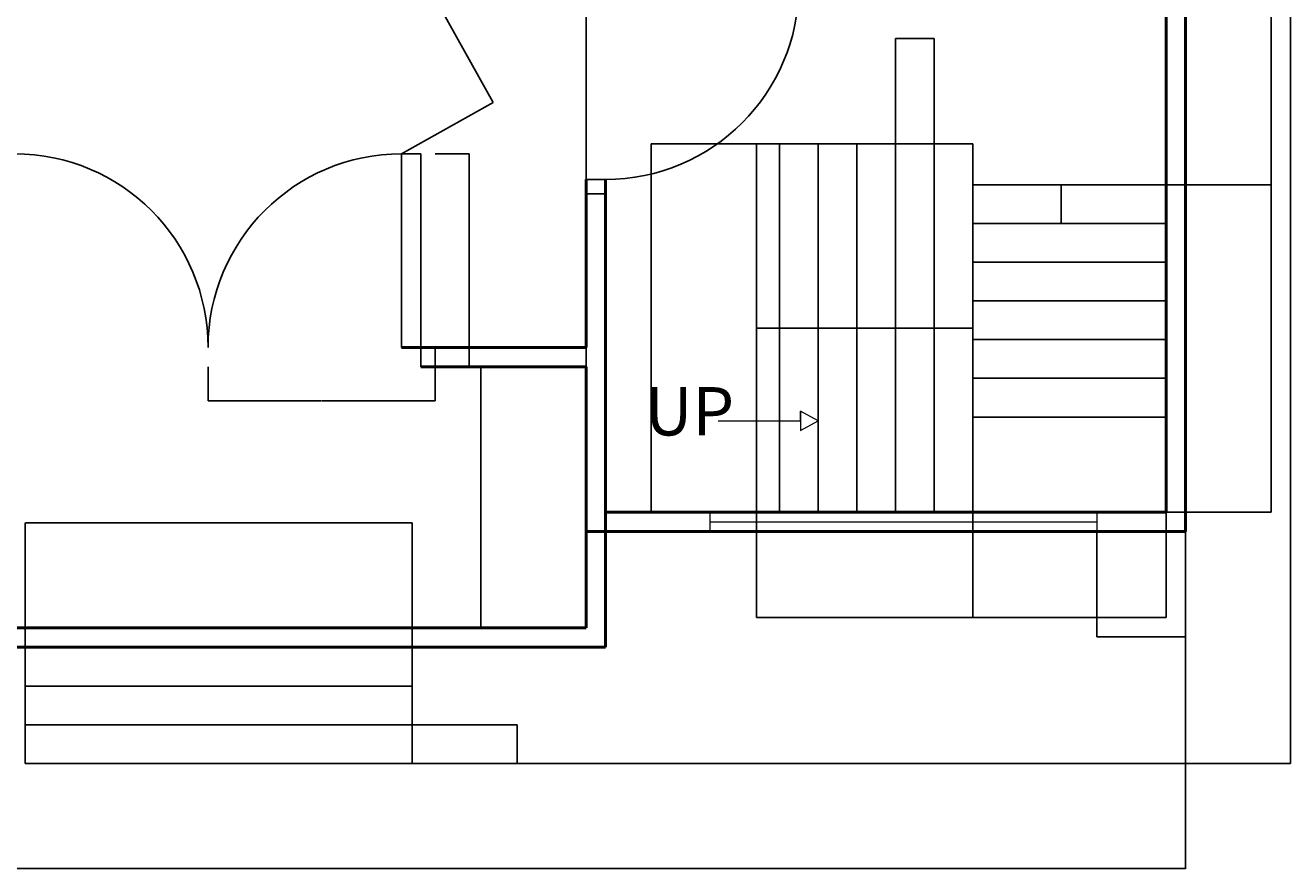
# Model space of a CAD drawing. Units: millimetres. Extents: x 1584 to 12772, y -932 to 10602.
# Tile 2 of 4: x 6228 to 12772, y -932 to 3427. Entities that reach past the tile are written whole.
import ezdxf

# ---------------------------------------------------------------- set-up
doc = ezdxf.new("R2010")
doc.units = ezdxf.units.MM
for name, color, linetype, lineweight in [('A-ANNO-DIMS', 2, 'Continuous', 18), ('A-ANNO-SYMB', 7, 'Continuous', 18), ('A-ANNO-TEXT', 7, 'Continuous', 25), ('A-DOOR', 3, 'Continuous', 25), ('A-FLOR-STRS', 7, 'Continuous', 25), ('A-GLAZ', 4, 'Continuous', 18), ('A-WALL', 7, 'Continuous', 50)]:
    doc.layers.add(name, color=color, linetype=linetype, lineweight=lineweight)
doc.styles.get("Standard").update_dxf_attribs({"font": 'arial.ttf'})
doc.dimstyles.get("Standard").update_dxf_attribs({"dimtxt": 0.18, "dimasz": 0.18, "dimexe": 0.18, "dimexo": 0.0625, "dimgap": 0.09, "dimtad": 0, "dimtih": 1, "dimtoh": 1, "dimdec": 4, "dimzin": 0, "dimdsep": 46, "dimtxsty": 'Standard', "dimcen": 0.09, "dimadec": 0, "dimazin": 0, "dimtfac": 1, "dimtdec": 4, "dimtofl": 0, "dimtmove": 0, "dimatfit": 3, "dimfxl": 1, "dimtolj": 1, "dimtzin": 0, "dimarcsym": 0})

# ---------------------------------------------------------------- blocks, each defined once
blk = doc.blocks.new('DOOR-SINGLE-1000')
for p, q in [((1000, 1174.2), (1000, 1248.4)), ((1000, 1248.4), (1100, 1248.4)), ((1100, 1248.4), (1100, 1174.2)), ((1000, 1174.2), (0, 1174.2)), ((0, 1174.2), (0, 1074.2)), ((1000, 1074.2), (1000, 1174.2)), ((1100, 1174.2), (1000, 1174.2)), ((0, 1074.2), (1000, 1074.2)), ((1000, 0), (1000, 74.2)), ((1000, 74.2), (1100, 74.2)), ((1100, 74.2), (1100, 0)), ((1100, 0), (1000, 0))]:
    blk.add_line(p, q)
blk.add_arc((1000, 1074.2), 1000, 180, 270)
blk = doc.blocks.new('DOOR-ENTRY-LEAF-1000')
for p, q in [((1100, 1100), (1000, 1100)), ((1000, 1100), (1000, 100)), ((1100, 100), (1100, 1100)), ((1000, 100), (1100, 100)), ((1100, 100), (1174.2, 100)), ((1100, 0), (1100, 100)), ((1174.2, 100), (1174.2, 0)), ((1174.2, 0), (1100, 0))]:
    blk.add_line(p, q)
blk.add_arc((1000, 100), 1000, 90, 180)
blk = doc.blocks.new('WIN-2000')
for p, q in [((0, 100), (2000, 100)), ((0, 0), (0, 100)), ((2000, 100), (2000, 0)), ((0, 50), (2000, 50)), ((2000, 0), (0, 0))]:
    blk.add_line(p, q)
blk = doc.blocks.new('*D22')
at = {"layer": 'A-ANNO-DIMS', "color": 0, "lineweight": -2, "transparency": 16777216}
for p, q in [((7172.8, 1662.3), (7172.8, 1486.1)), ((8347, 1662.3), (8347, 1486.1)), ((7173, 1486.2), (7758.4, 1486.2)), ((8346.8, 1486.2), (7761.4, 1486.2))]:
    blk.add_line(p, q, dxfattribs=at)
at = {"layer": 'A-ANNO-DIMS', "color": 0, "transparency": 16777216}
for points in [[(7173, 1486.3), (7173, 1486.2), (7172.8, 1486.2)], [(8346.8, 1486.3), (8346.8, 1486.2), (8347, 1486.2)]]:
    blk.add_solid(points, dxfattribs=at)
at = {"layer": 'Defpoints', "color": 0, "transparency": 16777216}
for p in [(7172.8, 1662.4), (8347, 1662.4), (8347, 1486.2)]:
    blk.add_point(p, dxfattribs=at)
at = {"layer": 'A-ANNO-DIMS', "color": 0, "transparency": 16777216, "insert": (7759.9, 1486.2), "char_height": 0.18, "attachment_point": 5}
blk.add_mtext('\\A1;ENTRY LEAF 1174 TYP.', dxfattribs=at)
blk = doc.blocks.new('*D23')
at = {"layer": 'A-ANNO-DIMS', "color": 0, "lineweight": -2, "transparency": 16777216}
for p, q in [((8347.1, 2762.4), (8523.3, 2762.4)), ((8523.2, 2762.2), (8523.2, 2212.5)), ((8523.2, 1662.5), (8523.2, 2212.2)), ((8347.1, 1662.4), (8523.3, 1662.4))]:
    blk.add_line(p, q, dxfattribs=at)
at = {"layer": 'A-ANNO-DIMS', "color": 0, "transparency": 16777216}
for points in [[(8523.1, 2762.2), (8523.2, 2762.2), (8523.2, 2762.4)], [(8523.1, 1662.5), (8523.2, 1662.5), (8523.2, 1662.4)]]:
    blk.add_solid(points, dxfattribs=at)
at = {"layer": 'Defpoints', "color": 0, "transparency": 16777216}
for p in [(8347, 2762.4), (8523.2, 2762.4), (8347, 1662.4)]:
    blk.add_point(p, dxfattribs=at)
at = {"layer": 'A-ANNO-DIMS', "color": 0, "transparency": 16777216, "insert": (8523.2, 2212.4), "char_height": 0.18, "attachment_point": 5}
blk.add_mtext('\\A1;1100 TYP.', dxfattribs=at)
blk = doc.blocks.new('*D36')
at = {"layer": 'A-ANNO-DIMS', "color": 0, "lineweight": -2, "transparency": 16777216}
for p, q in [((2127.8, 810.1), (2127.8, -931.5)), ((12227.8, 810.1), (12227.8, -931.5)), ((2128, -931.3), (7177.4, -931.3)), ((12227.7, -931.3), (7178.3, -931.3))]:
    blk.add_line(p, q, dxfattribs=at)
at = {"layer": 'A-ANNO-DIMS', "color": 0, "transparency": 16777216}
for points in [[(2128, -931.3), (2128, -931.4), (2127.8, -931.3)], [(12227.7, -931.3), (12227.7, -931.4), (12227.8, -931.3)]]:
    blk.add_solid(points, dxfattribs=at)
at = {"layer": 'Defpoints', "color": 0, "transparency": 16777216}
for p in [(2127.8, 810.2), (12227.8, 810.2), (12227.8, -931.3)]:
    blk.add_point(p, dxfattribs=at)
at = {"layer": 'A-ANNO-DIMS', "color": 0, "transparency": 16777216, "insert": (7177.8, -931.3), "char_height": 0.18, "attachment_point": 5}
blk.add_mtext('\\A1;10100', dxfattribs=at)
blk = doc.blocks.new('*D37')
at = {"layer": 'A-ANNO-DIMS', "color": 0, "lineweight": -2, "transparency": 16777216}
for p, q in [((12227.9, 9910.2), (12771.7, 9910.2)), ((12771.5, 9910), (12771.5, 4761.5)), ((12771.5, -387.5), (12771.5, 4761.1)), ((8227.9, -387.6), (12771.7, -387.6))]:
    blk.add_line(p, q, dxfattribs=at)
at = {"layer": 'A-ANNO-DIMS', "color": 0, "transparency": 16777216}
for points in [[(12771.5, 9910), (12771.6, 9910), (12771.5, 9910.2)], [(12771.5, -387.5), (12771.6, -387.5), (12771.5, -387.6)]]:
    blk.add_solid(points, dxfattribs=at)
at = {"layer": 'Defpoints', "color": 0, "transparency": 16777216}
for p in [(12227.8, 9910.2), (12771.5, 9910.2), (8227.8, -387.6)]:
    blk.add_point(p, dxfattribs=at)
at = {"layer": 'A-ANNO-DIMS', "color": 0, "transparency": 16777216, "insert": (12771.5, 4761.3), "char_height": 0.18, "attachment_point": 5}
blk.add_mtext('\\A1;10298', dxfattribs=at)
blk = doc.blocks.new('*D41')
at = {"layer": 'A-ANNO-DIMS', "color": 0, "lineweight": -2, "transparency": 16777216}
for p, q in [((12127.9, 4010.2), (12671.7, 4010.2)), ((12671.5, 4010), (12671.5, 3306.6)), ((12671.5, 2602.8), (12671.5, 3306.2)), ((12127.9, 2602.6), (12671.7, 2602.6))]:
    blk.add_line(p, q, dxfattribs=at)
at = {"layer": 'A-ANNO-DIMS', "color": 0, "transparency": 16777216}
for points in [[(12671.5, 4010), (12671.6, 4010), (12671.5, 4010.2)], [(12671.5, 2602.8), (12671.6, 2602.8), (12671.5, 2602.6)]]:
    blk.add_solid(points, dxfattribs=at)
at = {"layer": 'Defpoints', "color": 0, "transparency": 16777216}
for p in [(12127.8, 4010.2), (12127.8, 2602.6), (12671.5, 2602.6)]:
    blk.add_point(p, dxfattribs=at)
at = {"layer": 'A-ANNO-DIMS', "color": 0, "transparency": 16777216, "insert": (12671.5, 3306.4), "char_height": 0.18, "attachment_point": 5}
blk.add_mtext('\\A1;1407.6', dxfattribs=at)
blk = doc.blocks.new('*D44')
at = {"layer": 'A-ANNO-DIMS', "color": 0, "lineweight": -2, "transparency": 16777216}
for p, q in [((5227.8, 312.4), (5227.8, 10454.1)), ((5228, 10453.9), (7177.5, 10453.9)), ((9127.7, 10453.9), (7178.2, 10453.9)), ((9127.8, 312.4), (9127.8, 10454.1))]:
    blk.add_line(p, q, dxfattribs=at)
at = {"layer": 'A-ANNO-DIMS', "color": 0, "transparency": 16777216}
for points in [[(5228, 10453.9), (5228, 10453.9), (5227.8, 10453.9)], [(9127.7, 10453.9), (9127.7, 10453.9), (9127.8, 10453.9)]]:
    blk.add_solid(points, dxfattribs=at)
at = {"layer": 'Defpoints', "color": 0, "transparency": 16777216}
for p in [(9127.8, 10453.9), (5227.8, 312.4), (9127.8, 312.4)]:
    blk.add_point(p, dxfattribs=at)
at = {"layer": 'A-ANNO-DIMS', "color": 0, "transparency": 16777216, "insert": (7177.8, 10453.9), "char_height": 0.18, "attachment_point": 5}
blk.add_mtext('\\A1;3900', dxfattribs=at)
blk = doc.blocks.new('*D46')
at = {"layer": 'A-ANNO-DIMS', "color": 0, "lineweight": -2, "transparency": 16777216}
for p, q in [((9127.8, 1662.4), (8584, 1662.4)), ((8584.1, 1662.2), (8584.1, 987.5)), ((8584.1, 312.5), (8584.1, 987.2)), ((9127.8, 312.4), (8584, 312.4))]:
    blk.add_line(p, q, dxfattribs=at)
at = {"layer": 'A-ANNO-DIMS', "color": 0, "transparency": 16777216}
for points in [[(8584.1, 1662.2), (8584.2, 1662.2), (8584.1, 1662.4)], [(8584.1, 312.5), (8584.2, 312.5), (8584.1, 312.4)]]:
    blk.add_solid(points, dxfattribs=at)
at = {"layer": 'Defpoints', "color": 0, "transparency": 16777216}
for p in [(8584.1, 1662.4), (9127.8, 1662.4), (9127.8, 312.4)]:
    blk.add_point(p, dxfattribs=at)
at = {"layer": 'A-ANNO-DIMS', "color": 0, "transparency": 16777216, "insert": (8584.1, 987.4), "char_height": 0.18, "attachment_point": 5}
blk.add_mtext('\\A1;1350', dxfattribs=at)
blk = doc.blocks.new('*D47')
at = {"layer": 'A-ANNO-DIMS', "color": 0, "lineweight": -2, "transparency": 16777216}
for p, q in [((6227.83323, 312.424388), (6227.83323, 856.241888)), ((6228.01323, 856.061888), (7227.47323, 856.061888)), ((8227.65323, 856.061888), (7228.19323, 856.061888)), ((8227.83323, 312.424388), (8227.83323, 856.241888))]:
    blk.add_line(p, q, dxfattribs=at)
at = {"layer": 'A-ANNO-DIMS', "color": 0, "transparency": 16777216}
for points in [[(6228.01323, 856.091888), (6228.01323, 856.031888), (6227.83323, 856.061888)], [(8227.65323, 856.091888), (8227.65323, 856.031888), (8227.83323, 856.061888)]]:
    blk.add_solid(points, dxfattribs=at)
at = {"layer": 'Defpoints', "color": 0, "transparency": 16777216}
for p in [(8227.83323, 856.061888), (6227.83323, 312.361888), (8227.83323, 312.361888)]:
    blk.add_point(p, dxfattribs=at)
at = {"layer": 'A-ANNO-DIMS', "color": 0, "transparency": 16777216, "insert": (7227.83323, 856.061888), "char_height": 0.18, "attachment_point": 5}
blk.add_mtext('\\A1;2000', dxfattribs=at)
blk = doc.blocks.new('*D55')
at = {"layer": 'A-ANNO-DIMS', "color": 0, "lineweight": -2, "transparency": 16777216}
for p, q in [((11769.6, 810.1), (11769.6, 266.3)), ((12227.8, 810.1), (12227.8, 266.3)), ((11769.7, 266.5), (11998.3, 266.5)), ((12227.7, 266.5), (11999.1, 266.5))]:
    blk.add_line(p, q, dxfattribs=at)
at = {"layer": 'A-ANNO-DIMS', "color": 0, "transparency": 16777216}
for points in [[(11769.7, 266.5), (11769.7, 266.5), (11769.6, 266.5)], [(12227.7, 266.5), (12227.7, 266.5), (12227.8, 266.5)]]:
    blk.add_solid(points, dxfattribs=at)
at = {"layer": 'Defpoints', "color": 0, "transparency": 16777216}
for p in [(11769.6, 810.2), (12227.8, 810.2), (11769.6, 266.5)]:
    blk.add_point(p, dxfattribs=at)
at = {"layer": 'A-ANNO-DIMS', "color": 0, "transparency": 16777216, "insert": (11998.7, 266.5), "char_height": 0.18, "attachment_point": 5}
blk.add_mtext('\\A1;458.3', dxfattribs=at)
blk = doc.blocks.new('*D61')
at = {"layer": 'A-ANNO-DIMS', "color": 0, "lineweight": -2, "transparency": 16777216}
for p, q in [((11127.8, 910.1), (11127.8, 366.3)), ((12127.8, 910.1), (12127.8, 366.3)), ((11128, 366.5), (11627.5, 366.5)), ((12127.7, 366.5), (11628.2, 366.5))]:
    blk.add_line(p, q, dxfattribs=at)
at = {"layer": 'A-ANNO-DIMS', "color": 0, "transparency": 16777216}
for points in [[(11128, 366.5), (11128, 366.5), (11127.8, 366.5)], [(12127.7, 366.5), (12127.7, 366.5), (12127.8, 366.5)]]:
    blk.add_solid(points, dxfattribs=at)
at = {"layer": 'Defpoints', "color": 0, "transparency": 16777216}
for p in [(11127.8, 910.2), (12127.8, 910.2), (11127.8, 366.5)]:
    blk.add_point(p, dxfattribs=at)
at = {"layer": 'A-ANNO-DIMS', "color": 0, "transparency": 16777216, "insert": (11627.8, 366.5), "char_height": 0.18, "attachment_point": 5}
blk.add_mtext('\\A1;1000', dxfattribs=at)
blk = doc.blocks.new('*D62')
at = {"layer": 'A-ANNO-DIMS', "color": 0, "lineweight": -2, "transparency": 16777216}
for p, q in [((10008.6, 910.1), (10008.6, 366.3)), ((11127.8, 910.1), (11127.8, 366.3)), ((10008.8, 366.5), (10567.8, 366.5)), ((11127.7, 366.5), (10568.7, 366.5))]:
    blk.add_line(p, q, dxfattribs=at)
at = {"layer": 'A-ANNO-DIMS', "color": 0, "transparency": 16777216}
for points in [[(10008.8, 366.5), (10008.8, 366.5), (10008.6, 366.5)], [(11127.7, 366.5), (11127.7, 366.5), (11127.8, 366.5)]]:
    blk.add_solid(points, dxfattribs=at)
at = {"layer": 'Defpoints', "color": 0, "transparency": 16777216}
for p in [(10008.6, 910.2), (11127.8, 910.2), (10008.6, 366.5)]:
    blk.add_point(p, dxfattribs=at)
at = {"layer": 'A-ANNO-DIMS', "color": 0, "transparency": 16777216, "insert": (10568.2, 366.5), "char_height": 0.18, "attachment_point": 5}
blk.add_mtext('\\A1;1119.2', dxfattribs=at)
blk = doc.blocks.new('*D63')
at = {"layer": 'A-ANNO-DIMS', "color": 0, "lineweight": -2, "transparency": 16777216}
for p, q in [((10008.6, 2815.1), (9464.7, 2815.1)), ((9464.9, 2814.9), (9464.9, 1862.8)), ((9464.9, 910.4), (9464.9, 1862.4)), ((10008.6, 910.2), (9464.7, 910.2))]:
    blk.add_line(p, q, dxfattribs=at)
at = {"layer": 'A-ANNO-DIMS', "color": 0, "transparency": 16777216}
for points in [[(9464.9, 2814.9), (9464.9, 2814.9), (9464.9, 2815.1)], [(9464.9, 910.4), (9464.9, 910.4), (9464.9, 910.2)]]:
    blk.add_solid(points, dxfattribs=at)
at = {"layer": 'Defpoints', "color": 0, "transparency": 16777216}
for p in [(9464.9, 2815.1), (10008.6, 2815.1), (10008.6, 910.2)]:
    blk.add_point(p, dxfattribs=at)
at = {"layer": 'A-ANNO-DIMS', "color": 0, "transparency": 16777216, "insert": (9464.9, 1862.6), "char_height": 0.18, "attachment_point": 5}
blk.add_mtext('\\A1;1905', dxfattribs=at)
blk = doc.blocks.new('*D64')
at = {"layer": 'A-ANNO-DIMS', "color": 0, "lineweight": -2, "transparency": 16777216}
for p, q in [((12127.8, 2602.6), (11584, 2602.6)), ((11584.1, 2602.4), (11584.1, 2502.8)), ((11584.1, 2402.8), (11584.1, 2502.4)), ((12127.8, 2402.6), (11584, 2402.6))]:
    blk.add_line(p, q, dxfattribs=at)
at = {"layer": 'A-ANNO-DIMS', "color": 0, "transparency": 16777216}
for points in [[(11584.1, 2602.4), (11584.2, 2602.4), (11584.1, 2602.6)], [(11584.1, 2402.8), (11584.2, 2402.8), (11584.1, 2402.6)]]:
    blk.add_solid(points, dxfattribs=at)
at = {"layer": 'Defpoints', "color": 0, "transparency": 16777216}
for p in [(11584.1, 2602.6), (12127.8, 2602.6), (12127.8, 2402.6)]:
    blk.add_point(p, dxfattribs=at)
at = {"layer": 'A-ANNO-DIMS', "color": 0, "transparency": 16777216, "insert": (11584.1, 2502.6), "char_height": 0.18, "attachment_point": 5}
blk.add_mtext('\\A1;200', dxfattribs=at)
blk = doc.blocks.new('*D73')
at = {"layer": 'A-ANNO-DIMS', "color": 0, "lineweight": -2, "transparency": 16777216}
for p, q in [((7452.4, 4053), (7927.2, 4318.1)), ((7927.2, 4317.8), (8287.2, 3672.9)), ((8647.5, 3027.5), (8287.4, 3672.5)), ((8172.9, 2762.4), (8647.7, 3027.5))]:
    blk.add_line(p, q, dxfattribs=at)
at = {"layer": 'A-ANNO-DIMS', "color": 0, "transparency": 16777216}
for points in [[(7927.2, 4317.8), (7927.1, 4317.8), (7927.1, 4318)], [(8647.5, 3027.6), (8647.4, 3027.5), (8647.6, 3027.4)]]:
    blk.add_solid(points, dxfattribs=at)
at = {"layer": 'Defpoints', "color": 0, "transparency": 16777216}
for p in [(7452.3, 4053), (8647.6, 3027.4), (8172.8, 2762.4)]:
    blk.add_point(p, dxfattribs=at)
at = {"layer": 'A-ANNO-DIMS', "color": 0, "transparency": 16777216, "insert": (8287.3, 3672.7), "char_height": 0.18, "attachment_point": 5}
blk.add_mtext('\\A1;1478', dxfattribs=at)
blk = doc.blocks.new('*D77')
at = {"layer": 'A-ANNO-DIMS', "color": 0, "lineweight": -2, "transparency": 16777216}
for p, q in [((10727.8, 2815.1), (10727.8, 3358.9)), ((10728, 3358.8), (10827.5, 3358.8)), ((10927.7, 3358.8), (10828.1, 3358.8)), ((10927.8, 2815.1), (10927.8, 3358.9))]:
    blk.add_line(p, q, dxfattribs=at)
at = {"layer": 'A-ANNO-DIMS', "color": 0, "transparency": 16777216}
for points in [[(10728, 3358.8), (10728, 3358.7), (10727.8, 3358.8)], [(10927.7, 3358.8), (10927.7, 3358.7), (10927.8, 3358.8)]]:
    blk.add_solid(points, dxfattribs=at)
at = {"layer": 'Defpoints', "color": 0, "transparency": 16777216}
for p in [(10927.8, 3358.8), (10727.8, 2815.1), (10927.8, 2815.1)]:
    blk.add_point(p, dxfattribs=at)
at = {"layer": 'A-ANNO-DIMS', "color": 0, "transparency": 16777216, "insert": (10827.8, 3358.8), "char_height": 0.18, "attachment_point": 5}
blk.add_mtext('\\A1;200', dxfattribs=at)
blk = doc.blocks.new('*D78')
at = {"layer": 'A-ANNO-DIMS', "color": 0, "lineweight": -2, "transparency": 16777216}
for p, q in [((12127.9, 2602.6), (12671.7, 2602.6)), ((12671.5, 2602.4), (12671.5, 1756.6)), ((12671.5, 910.4), (12671.5, 1756.2)), ((12127.9, 910.2), (12671.7, 910.2))]:
    blk.add_line(p, q, dxfattribs=at)
at = {"layer": 'A-ANNO-DIMS', "color": 0, "transparency": 16777216}
for points in [[(12671.5, 2602.4), (12671.6, 2602.4), (12671.5, 2602.6)], [(12671.5, 910.4), (12671.6, 910.4), (12671.5, 910.2)]]:
    blk.add_solid(points, dxfattribs=at)
at = {"layer": 'Defpoints', "color": 0, "transparency": 16777216}
for p in [(12127.8, 2602.6), (12127.8, 910.2), (12671.5, 910.2)]:
    blk.add_point(p, dxfattribs=at)
at = {"layer": 'A-ANNO-DIMS', "color": 0, "transparency": 16777216, "insert": (12671.5, 1756.4), "char_height": 0.18, "attachment_point": 5}
blk.add_mtext('\\A1;1692.4', dxfattribs=at)
blk = doc.blocks.new('*D79')
at = {"layer": 'A-ANNO-DIMS', "color": 0, "lineweight": -2, "transparency": 16777216}
for p, q in [((8227.9, -187.6), (8771.7, -187.6)), ((8771.5, -187.8), (8771.5, -287.5)), ((8771.5, -387.5), (8771.5, -287.8)), ((8227.9, -387.6), (8771.7, -387.6))]:
    blk.add_line(p, q, dxfattribs=at)
at = {"layer": 'A-ANNO-DIMS', "color": 0, "transparency": 16777216}
for points in [[(8771.5, -187.8), (8771.6, -187.8), (8771.5, -187.6)], [(8771.5, -387.5), (8771.6, -387.5), (8771.5, -387.6)]]:
    blk.add_solid(points, dxfattribs=at)
at = {"layer": 'Defpoints', "color": 0, "transparency": 16777216}
for p in [(8227.8, -187.6), (8227.8, -387.6), (8771.5, -387.6)]:
    blk.add_point(p, dxfattribs=at)
at = {"layer": 'A-ANNO-DIMS', "color": 0, "transparency": 16777216, "insert": (8771.5, -287.6), "char_height": 0.18, "attachment_point": 5}
blk.add_mtext('\\A1;200', dxfattribs=at)

msp = doc.modelspace()

# ---------------------------------------------------------------- linework, layer by layer
at = {"layer": 'A-ANNO-SYMB'}
for p, q in [((9811.093, 1382.479), (10236.082, 1382.479)), ((10236.082, 1407.479), (10236.082, 1432.479)), ((10236.082, 1432.479), (10236.082, 1382.479)), ((10327.833, 1382.479), (10236.082, 1432.479)), ((10236.082, 1382.479), (10236.082, 1407.479)), ((10236.082, 1382.479), (10236.082, 1332.479)), ((10236.082, 1332.479), (10327.833, 1382.479))]:
    msp.add_line(p, q, dxfattribs=at)
at = {"layer": 'A-FLOR-STRS'}
for p, q in [((11127.833, 2815.06), (10008.619, 2815.06)), ((10008.619, 2815.06), (10008.619, 910.181)), ((10127.833, 2602.614), (10127.833, 2815.06)), ((10327.833, 2602.614), (10327.833, 2815.06)), ((10527.833, 2602.614), (10527.833, 2815.06)), ((10727.833, 2602.614), (10727.833, 2815.06)), ((10927.833, 2602.614), (10927.833, 2815.06)), ((11127.833, 2602.614), (11127.833, 2815.06)), ((10127.833, 910.181), (10127.833, 2602.614)), ((10327.833, 910.181), (10327.833, 2602.614)), ((10527.833, 910.181), (10527.833, 2602.614)), ((10727.833, 910.181), (10727.833, 2602.614)), ((10927.833, 910.181), (10927.833, 2602.614)), ((11127.833, 910.181), (11127.833, 2602.614)), ((11127.833, 2602.614), (12127.833, 2602.614)), ((12127.833, 2602.614), (11127.833, 2602.614)), ((12127.833, 2402.614), (11127.833, 2402.614)), ((12127.833, 2202.614), (11127.833, 2202.614)), ((12127.833, 2002.614), (11127.833, 2002.614)), ((10008.619, 1862.62), (11127.833, 1862.62)), ((12127.833, 1802.614), (11127.833, 1802.614)), ((12127.833, 1602.614), (11127.833, 1602.614)), ((12127.833, 1402.614), (11127.833, 1402.614)), ((12127.833, 910.181), (11127.833, 910.181)), ((6227.833, -387.638), (6227.833, 312.362)), ((8227.833, -387.638), (8227.833, 312.362)), ((7227.833, 12.362), (6227.833, 12.362)), ((8227.833, 12.362), (7227.833, 12.362)), ((7227.833, -187.638), (6227.833, -187.638)), ((8227.833, -187.638), (7227.833, -187.638)), ((7227.833, -387.638), (6227.833, -387.638)), ((7227.833, -387.638), (7727.833, -387.638)), ((8227.833, -387.638), (7227.833, -387.638)), ((7727.833, -387.638), (8227.833, -387.638))]:
    msp.add_line(p, q, dxfattribs=at)
at = {"layer": 'A-WALL'}
for p, q in [((12227.833, 9910.181), (12227.833, 810.181)), ((12127.833, 4010.181), (12127.833, 910.181)), ((9127.833, 2630.192), (9127.833, 2410.181)), ((9227.833, 2630.192), (9227.833, 910.181)), ((9127.833, 2410.181), (9127.833, 2310.181)), ((9127.833, 2310.181), (9127.833, 1762.362)), ((8172.821, 1762.362), (9127.833, 1762.362)), ((8272.821, 1662.362), (9127.833, 1662.362)), ((9127.833, 1662.362), (9127.833, 910.181)), ((9127.833, 910.181), (9127.833, 312.362)), ((9227.833, 910.181), (12127.833, 910.181)), ((9227.833, 212.362), (9227.833, 910.181)), ((9127.833, 810.181), (12227.833, 810.181)), ((5227.833, 312.362), (9127.833, 312.362)), ((9127.833, 212.362), (5127.833, 212.362)), ((5227.833, 212.362), (9227.833, 212.362))]:
    msp.add_line(p, q, dxfattribs=at)

# ---------------------------------------------------------------- block references
at = {"layer": 'A-DOOR', "extrusion": (0, 0, -1), "zscale": -1}
for name, p in [('DOOR-SINGLE-1000', (-10227.833, 2555.992)), ('DOOR-ENTRY-LEAF-1000', (-7172.82, 1662.362))]:
    msp.add_blockref(name, p, dxfattribs=at)
at = {"layer": 'A-DOOR'}
msp.add_blockref('DOOR-ENTRY-LEAF-1000', (7172.821, 1662.362), dxfattribs=at)
at = {"layer": 'A-GLAZ'}
msp.add_blockref('WIN-2000', (9769.557, 810.181), dxfattribs=at)

# ---------------------------------------------------------------- texts
at = {"layer": 'A-ANNO-TEXT', "insert": (9432.028, 1557.338), "char_height": 250, "attachment_point": 1}
msp.add_mtext_dynamic_manual_height_columns('UP', width=365.75146, gutter_width=12.5, heights=[0], dxfattribs=at)

# ---------------------------------------------------------------- dimensions: what is measured, and where the dimension line sits
at = {"layer": 'A-ANNO-DIMS'}
for base, p1, p2, picture, middle in [((9127.833, 10453.881), (5227.833, 312.362), (9127.833, 312.362), '*D44', (7177.833, 10453.881)), ((10927.833, 3358.76), (10727.833, 2815.06), (10927.833, 2815.06), '*D77', (10827.833, 3358.76)), ((8227.833, 856.062), (6227.833, 312.362), (8227.833, 312.362), '*D47', (7227.833, 856.062)), ((12227.833, -931.338), (2127.833, 810.181), (12227.833, 810.181), '*D36', (7177.833, -931.338))]:
    dim = msp.add_linear_dim(base=base, p1=p1, p2=p2, dimstyle='Standard', override={"dimdec": 0, "dimlfac": 1, "dimrnd": 0, "dimzin": 0, "dimdsep": 46, "dimlunit": 2}, dxfattribs=at)
    dim.commit()
    dim.dimension.update_dxf_attribs({"geometry": picture, "text_midpoint": middle})
for base, p1, p2, angle, override, picture, middle in [((12771.533, 9910.181), (8227.833, -387.638), (12227.833, 9910.181), 90, {"dimdec": 0, "dimlfac": 1, "dimrnd": 0, "dimzin": 0, "dimdsep": 46, "dimlunit": 2}, '*D37', (12771.533, 4761.271)), ((8647.556, 3027.383), (7452.347, 4052.958), (8172.821, 2762.362), 299.1724058, {"dimdec": 0, "dimlfac": 1, "dimrnd": 0, "dimzin": 0, "dimdsep": 46, "dimlunit": 2}, '*D73', (8287.319, 3672.68)), ((12671.533, 2602.614), (12127.833, 4010.181), (12127.833, 2602.614), 270, {"dimdec": 1, "dimlfac": 1, "dimrnd": 0, "dimzin": 0, "dimdsep": 46, "dimlunit": 2}, '*D41', (12671.533, 3306.397)), ((9464.919, 2815.06), (10008.619, 910.181), (10008.619, 2815.06), 90, {"dimdec": 0, "dimlfac": 1, "dimrnd": 0, "dimzin": 0, "dimdsep": 46, "dimlunit": 2}, '*D63', (9464.919, 1862.62)), ((11584.133, 2602.614), (12127.833, 2402.614), (12127.833, 2602.614), 90, {"dimdec": 0, "dimlfac": 1, "dimrnd": 0, "dimzin": 0, "dimdsep": 46, "dimlunit": 2}, '*D64', (11584.133, 2502.614)), ((12671.533, 910.181), (12127.833, 2602.614), (12127.833, 910.181), 270, {"dimdec": 1, "dimlfac": 1, "dimrnd": 0, "dimzin": 0, "dimdsep": 46, "dimlunit": 2}, '*D78', (12671.533, 1756.397)), ((8584.133, 1662.362), (9127.833, 312.362), (9127.833, 1662.362), 90, {"dimdec": 0, "dimlfac": 1, "dimrnd": 0, "dimzin": 0, "dimdsep": 46, "dimlunit": 2}, '*D46', (8584.133, 987.362)), ((10008.619, 366.481), (11127.833, 910.181), (10008.619, 910.181), 180, {"dimdec": 1, "dimlfac": 1, "dimrnd": 0, "dimzin": 0, "dimdsep": 46, "dimlunit": 2}, '*D62', (10568.226, 366.481)), ((11127.833, 366.481), (12127.833, 910.181), (11127.833, 910.181), 180, {"dimdec": 0, "dimlfac": 1, "dimrnd": 0, "dimzin": 0, "dimdsep": 46, "dimlunit": 2}, '*D61', (11627.833, 366.481)), ((11769.557, 266.481), (12227.833, 810.181), (11769.557, 810.181), 180, {"dimdec": 1, "dimlfac": 1, "dimrnd": 0, "dimzin": 0, "dimdsep": 46, "dimlunit": 2}, '*D55', (11998.695, 266.481)), ((8771.533, -387.638), (8227.833, -187.638), (8227.833, -387.638), 270, {"dimdec": 0, "dimlfac": 1, "dimrnd": 0, "dimzin": 0, "dimdsep": 46, "dimlunit": 2}, '*D79', (8771.533, -287.638))]:
    dim = msp.add_linear_dim(base=base, p1=p1, p2=p2, angle=angle, dimstyle='Standard', override=override, dxfattribs=at)
    dim.commit()
    dim.dimension.update_dxf_attribs({"geometry": picture, "text_midpoint": middle})
dim = msp.add_linear_dim(base=(8523.151, 2762.362), p1=(8347.021, 1662.362), p2=(8347.021, 2762.362), angle=90, text='<> TYP.', dimstyle='Standard', override={"dimdec": 0, "dimlfac": 1, "dimrnd": 0, "dimzin": 0, "dimdsep": 46, "dimlunit": 2}, dxfattribs=at)
dim.commit()
dim.dimension.update_dxf_attribs({"geometry": '*D23', "text_midpoint": (8523.151, 2212.362)})
dim = msp.add_linear_dim(base=(8347.021, 1486.232), p1=(7172.821, 1662.362), p2=(8347.021, 1662.362), text='ENTRY LEAF <> TYP.', dimstyle='Standard', override={"dimdec": 0, "dimlfac": 1, "dimrnd": 0, "dimzin": 0, "dimdsep": 46, "dimlunit": 2}, dxfattribs=at)
dim.commit()
dim.dimension.update_dxf_attribs({"geometry": '*D22', "text_midpoint": (7759.921, 1486.232)})

doc.saveas('drawing.dxf')
